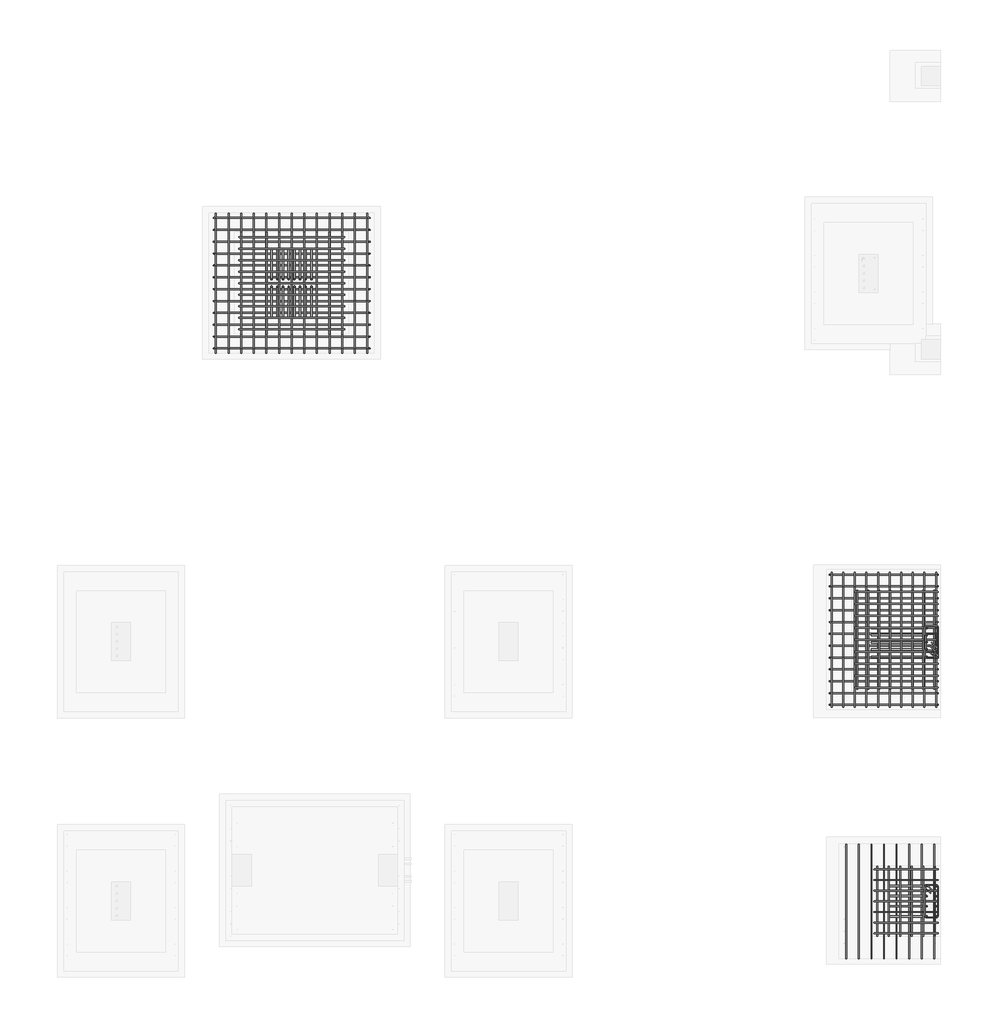
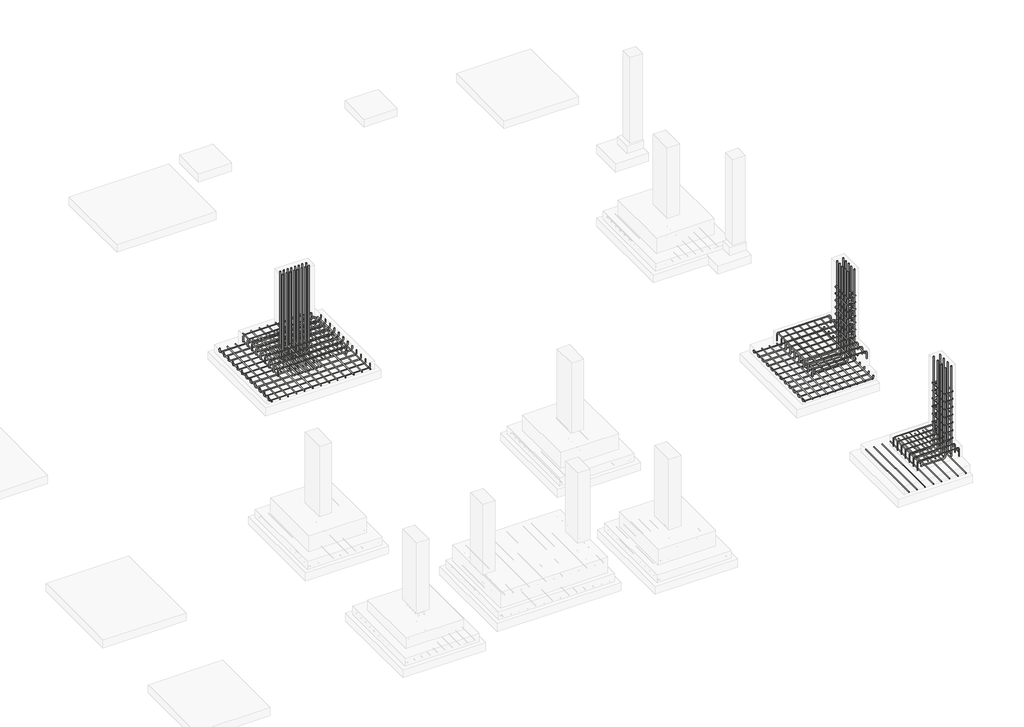
# One storey, part 5 of 6: 20 reinforcing bars.
"""IFC4 building model written with IfcOpenShell, lengths in millimetres."""

from ifc_helpers import new_model, si_unit, point, frame, origin, place, context, project, spatial, polyline, circle_curve, trimmed, segment, composite_curve, source, transform, mapped, element, save
from ifc_brep_helpers import swept_disk

model = new_model("IFC4")

# Units and contexts
model_context = context("Model", 3, world=origin())
ifc_project = project(units=[si_unit("LENGTHUNIT", "METRE", prefix="MILLI")], contexts=[model_context])

# Site, building, storey
site = spatial("IfcSite", under=ifc_project)
building = spatial("IfcBuilding", under=site)
storey = spatial("IfcBuildingStorey", under=building, Elevation=-1828.8)

# Reinforcing bars
placement = place(None, origin())
reinforcing_bar_shape = source(origin(), model_context, "Body", "SolidModel", [
    swept_disk(composite_curve([segment(polyline([(5676850.791013, -3593831.6523052, -1801.3373708), (5676850.791013, -3595448.0523052, -1801.3373708)]), True, "CONTINUOUS")], self_intersect=False), 6.0),
])
element("IfcReinforcingBar", 1, at=placement, inside=storey, context=model_context, shape_type="MappedRepresentation", body=[
    mapped(reinforcing_bar_shape, transform((0.0, 0.0, 0.0), x_axis=(1.0, 0.0, 0.0), y_axis=(0.0, 1.0, 0.0), z_axis=(0.0, 0.0, 1.0))),
    mapped(reinforcing_bar_shape, transform((-139.1053792, 0.0, 0.0), x_axis=(1.0, 0.0, 0.0), y_axis=(0.0, 1.0, 0.0), z_axis=(0.0, 0.0, 1.0))),
    mapped(reinforcing_bar_shape, transform((-278.2107585, 0.0, 0.0), x_axis=(1.0, 0.0, 0.0), y_axis=(0.0, 1.0, 0.0), z_axis=(0.0, 0.0, 1.0))),
    mapped(reinforcing_bar_shape, transform((-417.3161377, 0.0, 0.0), x_axis=(1.0, 0.0, 0.0), y_axis=(0.0, 1.0, 0.0), z_axis=(0.0, 0.0, 1.0))),
    mapped(reinforcing_bar_shape, transform((-556.4215169, 0.0, 0.0), x_axis=(1.0, 0.0, 0.0), y_axis=(0.0, 1.0, 0.0), z_axis=(0.0, 0.0, 1.0))),
    mapped(reinforcing_bar_shape, transform((-695.5268961, 0.0, 0.0), x_axis=(1.0, 0.0, 0.0), y_axis=(0.0, 1.0, 0.0), z_axis=(0.0, 0.0, 1.0))),
    mapped(reinforcing_bar_shape, transform((-834.6322754, 0.0, 0.0), x_axis=(1.0, 0.0, 0.0), y_axis=(0.0, 1.0, 0.0), z_axis=(0.0, 0.0, 1.0))),
    mapped(reinforcing_bar_shape, transform((-973.7376546, 0.0, 0.0), x_axis=(1.0, 0.0, 0.0), y_axis=(0.0, 1.0, 0.0), z_axis=(0.0, 0.0, 1.0))),
    mapped(reinforcing_bar_shape, transform((-1112.8430338, 0.0, 0.0), x_axis=(1.0, 0.0, 0.0), y_axis=(0.0, 1.0, 0.0), z_axis=(0.0, 0.0, 1.0))),
    mapped(reinforcing_bar_shape, transform((-1251.9484131, 0.0, 0.0), x_axis=(1.0, 0.0, 0.0), y_axis=(0.0, 1.0, 0.0), z_axis=(0.0, 0.0, 1.0))),
])
reinforcing_bar_2_shape = source(origin(), model_context, "Body", "SolidModel", [
    swept_disk(composite_curve([segment(polyline([(5675879.3650571, -3595213.4523052, -1551.6), (5675879.3650571, -3595213.4523052, -1437.6)]), True, "CONTINUOUS"), segment(trimmed(circle_curve(frame((5675909.3650571, -3595213.4523052, -1437.6), z_axis=(0.0, 1.0, 0.0), x_axis=(-30.0, 0.0, 0.0)), 30.0), [point((5675879.3650571, -3595213.4523052, -1437.6))], [point((5675909.3650571, -3595213.4523052, -1407.6))], True, "CARTESIAN"), True, "CONTINUOUS"), segment(polyline([(5675909.3650571, -3595213.4523052, -1407.6), (5676844.1650571, -3595213.4523052, -1407.6)]), True, "CONTINUOUS"), segment(trimmed(circle_curve(frame((5676844.1650571, -3595213.4523052, -1437.6), z_axis=(0.0, 1.0, 0.0), x_axis=(0.0, 0.0, 30.0)), 30.0), [point((5676844.1650571, -3595213.4523052, -1407.6))], [point((5676874.1650571, -3595213.4523052, -1437.6))], True, "CARTESIAN"), True, "CONTINUOUS"), segment(polyline([(5676874.1650571, -3595213.4523052, -1437.6), (5676874.1650571, -3595213.4523052, -1551.6)]), True, "CONTINUOUS")], self_intersect=False), 6.0),
])
element("IfcReinforcingBar", 2, at=placement, inside=storey, context=model_context, shape_type="MappedRepresentation", body=[
    mapped(reinforcing_bar_2_shape, transform((0.0, 0.0, 0.0), x_axis=(1.0, 0.0, 0.0), y_axis=(0.0, 1.0, 0.0), z_axis=(0.0, 0.0, 1.0))),
    mapped(reinforcing_bar_2_shape, transform((0.0, 143.4, 0.0), x_axis=(1.0, 0.0, 0.0), y_axis=(0.0, 1.0, 0.0), z_axis=(0.0, 0.0, 1.0))),
    mapped(reinforcing_bar_2_shape, transform((0.0, 286.8, 0.0), x_axis=(1.0, 0.0, 0.0), y_axis=(0.0, 1.0, 0.0), z_axis=(0.0, 0.0, 1.0))),
    mapped(reinforcing_bar_2_shape, transform((0.0, 430.2, 0.0), x_axis=(1.0, 0.0, 0.0), y_axis=(0.0, 1.0, 0.0), z_axis=(0.0, 0.0, 1.0))),
    mapped(reinforcing_bar_2_shape, transform((0.0, 573.6, 0.0), x_axis=(1.0, 0.0, 0.0), y_axis=(0.0, 1.0, 0.0), z_axis=(0.0, 0.0, 1.0))),
    mapped(reinforcing_bar_2_shape, transform((0.0, 717.0, 0.0), x_axis=(1.0, 0.0, 0.0), y_axis=(0.0, 1.0, 0.0), z_axis=(0.0, 0.0, 1.0))),
    mapped(reinforcing_bar_2_shape, transform((0.0, 860.4, 0.0), x_axis=(1.0, 0.0, 0.0), y_axis=(0.0, 1.0, 0.0), z_axis=(0.0, 0.0, 1.0))),
    mapped(reinforcing_bar_2_shape, transform((0.0, 1003.8, 0.0), x_axis=(1.0, 0.0, 0.0), y_axis=(0.0, 1.0, 0.0), z_axis=(0.0, 0.0, 1.0))),
    mapped(reinforcing_bar_2_shape, transform((0.0, 1147.2, 0.0), x_axis=(1.0, 0.0, 0.0), y_axis=(0.0, 1.0, 0.0), z_axis=(0.0, 0.0, 1.0))),
])
reinforcing_bar_3_shape = source(origin(), model_context, "Body", "SolidModel", [
    swept_disk(composite_curve([segment(polyline([(5675905.090534, -3595232.9223129, -1420.5088801), (5675905.090534, -3594045.3578875, -1420.5088801)]), True, "CONTINUOUS")], self_intersect=False), 6.0),
])
element("IfcReinforcingBar", 3, at=placement, inside=storey, context=model_context, shape_type="MappedRepresentation", body=[
    mapped(reinforcing_bar_3_shape, transform((0.0, 0.0, 0.0), x_axis=(1.0, 0.0, 0.0), y_axis=(0.0, 1.0, 0.0), z_axis=(0.0, 0.0, 1.0))),
    mapped(reinforcing_bar_3_shape, transform((131.8407277, 0.0, 0.0), x_axis=(1.0, 0.0, 0.0), y_axis=(0.0, 1.0, 0.0), z_axis=(0.0, 0.0, 1.0))),
    mapped(reinforcing_bar_3_shape, transform((263.6814554, 0.0, 0.0), x_axis=(1.0, 0.0, 0.0), y_axis=(0.0, 1.0, 0.0), z_axis=(0.0, 0.0, 1.0))),
    mapped(reinforcing_bar_3_shape, transform((395.5221831, 0.0, 0.0), x_axis=(1.0, 0.0, 0.0), y_axis=(0.0, 1.0, 0.0), z_axis=(0.0, 0.0, 1.0))),
    mapped(reinforcing_bar_3_shape, transform((527.3629109, 0.0, 0.0), x_axis=(1.0, 0.0, 0.0), y_axis=(0.0, 1.0, 0.0), z_axis=(0.0, 0.0, 1.0))),
    mapped(reinforcing_bar_3_shape, transform((659.2036386, 0.0, 0.0), x_axis=(1.0, 0.0, 0.0), y_axis=(0.0, 1.0, 0.0), z_axis=(0.0, 0.0, 1.0))),
    mapped(reinforcing_bar_3_shape, transform((791.0443663, 0.0, 0.0), x_axis=(1.0, 0.0, 0.0), y_axis=(0.0, 1.0, 0.0), z_axis=(0.0, 0.0, 1.0))),
    mapped(reinforcing_bar_3_shape, transform((922.885094, 0.0, 0.0), x_axis=(1.0, 0.0, 0.0), y_axis=(0.0, 1.0, 0.0), z_axis=(0.0, 0.0, 1.0))),
])
reinforcing_bar_4_shape = source(origin(), model_context, "Body", "SolidModel", [
    swept_disk(composite_curve([segment(polyline([(5675574.5650571, -3593858.3316435, -1763.0663631), (5675574.5650571, -3593858.3316435, -1784.4413329)]), True, "CONTINUOUS"), segment(trimmed(circle_curve(frame((5675604.5650571, -3593858.3316435, -1784.4413329), z_axis=(0.0, -1.0, 0.0), x_axis=(-30.0, 0.0, 0.0)), 30.0), [point((5675574.5650571, -3593858.3316435, -1784.4413329))], [point((5675604.5650571, -3593858.3316435, -1814.4413329))], True, "CARTESIAN"), True, "CONTINUOUS"), segment(polyline([(5675604.5650571, -3593858.3316435, -1814.4413329), (5676844.1650571, -3593858.3316435, -1814.4413329)]), True, "CONTINUOUS"), segment(trimmed(circle_curve(frame((5676844.1650571, -3593858.3316435, -1784.4413329), z_axis=(0.0, -1.0, 0.0), x_axis=(0.0, 0.0, -30.0)), 30.0), [point((5676844.1650571, -3593858.3316435, -1814.4413329))], [point((5676874.1650571, -3593858.3316435, -1784.4413329))], True, "CARTESIAN"), True, "CONTINUOUS"), segment(polyline([(5676874.1650571, -3593858.3316435, -1784.4413329), (5676874.1650571, -3593858.3316435, -1763.0663631)]), True, "CONTINUOUS")], self_intersect=False), 6.0),
])
element("IfcReinforcingBar", 4, at=placement, inside=storey, context=model_context, shape_type="MappedRepresentation", body=[
    mapped(reinforcing_bar_4_shape, transform((0.0, 0.0, 0.0), x_axis=(1.0, 0.0, 0.0), y_axis=(0.0, 1.0, 0.0), z_axis=(0.0, 0.0, 1.0))),
    mapped(reinforcing_bar_4_shape, transform((0.0, -142.0493969, 0.0), x_axis=(1.0, 0.0, 0.0), y_axis=(0.0, 1.0, 0.0), z_axis=(0.0, 0.0, 1.0))),
    mapped(reinforcing_bar_4_shape, transform((0.0, -284.0987939, 0.0), x_axis=(1.0, 0.0, 0.0), y_axis=(0.0, 1.0, 0.0), z_axis=(0.0, 0.0, 1.0))),
    mapped(reinforcing_bar_4_shape, transform((0.0, -426.1481908, 0.0), x_axis=(1.0, 0.0, 0.0), y_axis=(0.0, 1.0, 0.0), z_axis=(0.0, 0.0, 1.0))),
    mapped(reinforcing_bar_4_shape, transform((0.0, -568.1975878, 0.0), x_axis=(1.0, 0.0, 0.0), y_axis=(0.0, 1.0, 0.0), z_axis=(0.0, 0.0, 1.0))),
    mapped(reinforcing_bar_4_shape, transform((0.0, -710.2469847, 0.0), x_axis=(1.0, 0.0, 0.0), y_axis=(0.0, 1.0, 0.0), z_axis=(0.0, 0.0, 1.0))),
    mapped(reinforcing_bar_4_shape, transform((0.0, -852.2963817, 0.0), x_axis=(1.0, 0.0, 0.0), y_axis=(0.0, 1.0, 0.0), z_axis=(0.0, 0.0, 1.0))),
    mapped(reinforcing_bar_4_shape, transform((0.0, -994.3457786, 0.0), x_axis=(1.0, 0.0, 0.0), y_axis=(0.0, 1.0, 0.0), z_axis=(0.0, 0.0, 1.0))),
    mapped(reinforcing_bar_4_shape, transform((0.0, -1136.3951756, 0.0), x_axis=(1.0, 0.0, 0.0), y_axis=(0.0, 1.0, 0.0), z_axis=(0.0, 0.0, 1.0))),
    mapped(reinforcing_bar_4_shape, transform((0.0, -1278.4445725, 0.0), x_axis=(1.0, 0.0, 0.0), y_axis=(0.0, 1.0, 0.0), z_axis=(0.0, 0.0, 1.0))),
    mapped(reinforcing_bar_4_shape, transform((0.0, -1420.4939694, 0.0), x_axis=(1.0, 0.0, 0.0), y_axis=(0.0, 1.0, 0.0), z_axis=(0.0, 0.0, 1.0))),
    mapped(reinforcing_bar_4_shape, transform((0.0, -1562.5433664, 0.0), x_axis=(1.0, 0.0, 0.0), y_axis=(0.0, 1.0, 0.0), z_axis=(0.0, 0.0, 1.0))),
])
reinforcing_bar_5_shape = source(origin(), model_context, "Body", "SolidModel", [
    swept_disk(composite_curve([segment(polyline([(5675774.6470228, -3597090.2875145, -1807.7638193), (5675774.6470228, -3598461.8875145, -1807.7638193)]), True, "CONTINUOUS")], self_intersect=False), 5.0),
])
element("IfcReinforcingBar", 5, at=placement, inside=storey, context=model_context, shape_type="MappedRepresentation", body=[
    mapped(reinforcing_bar_5_shape, transform((0.0, 0.0, 0.0), x_axis=(1.0, 0.0, 0.0), y_axis=(0.0, 1.0, 0.0), z_axis=(0.0, 0.0, 1.0))),
    mapped(reinforcing_bar_5_shape, transform((150.6667583, 0.0, 0.0), x_axis=(1.0, 0.0, 0.0), y_axis=(0.0, 1.0, 0.0), z_axis=(0.0, 0.0, 1.0))),
    mapped(reinforcing_bar_5_shape, transform((301.3335165, 0.0, 0.0), x_axis=(1.0, 0.0, 0.0), y_axis=(0.0, 1.0, 0.0), z_axis=(0.0, 0.0, 1.0))),
    mapped(reinforcing_bar_5_shape, transform((452.0002748, 0.0, 0.0), x_axis=(1.0, 0.0, 0.0), y_axis=(0.0, 1.0, 0.0), z_axis=(0.0, 0.0, 1.0))),
    mapped(reinforcing_bar_5_shape, transform((602.6670331, 0.0, 0.0), x_axis=(1.0, 0.0, 0.0), y_axis=(0.0, 1.0, 0.0), z_axis=(0.0, 0.0, 1.0))),
    mapped(reinforcing_bar_5_shape, transform((753.3337913, 0.0, 0.0), x_axis=(1.0, 0.0, 0.0), y_axis=(0.0, 1.0, 0.0), z_axis=(0.0, 0.0, 1.0))),
    mapped(reinforcing_bar_5_shape, transform((904.0005496, 0.0, 0.0), x_axis=(1.0, 0.0, 0.0), y_axis=(0.0, 1.0, 0.0), z_axis=(0.0, 0.0, 1.0))),
    mapped(reinforcing_bar_5_shape, transform((1054.6673079, 0.0, 0.0), x_axis=(1.0, 0.0, 0.0), y_axis=(0.0, 1.0, 0.0), z_axis=(0.0, 0.0, 1.0))),
])
reinforcing_bar_6_shape = source(origin(), model_context, "Body", "SolidModel", [
    swept_disk(composite_curve([segment(polyline([(5676875.1650571, -3597391.9875145, -1673.2), (5676875.1650571, -3597391.9875145, -1533.2)]), True, "CONTINUOUS"), segment(trimmed(circle_curve(frame((5676850.1650571, -3597391.9875145, -1533.2), z_axis=(0.0, -1.0, 0.0), x_axis=(25.0, 0.0, 0.0)), 25.0), [point((5676875.1650571, -3597391.9875145, -1533.2))], [point((5676850.1650571, -3597391.9875145, -1508.2))], True, "CARTESIAN"), True, "CONTINUOUS"), segment(polyline([(5676850.1650571, -3597391.9875145, -1508.2), (5676131.9650571, -3597391.9875145, -1508.2)]), True, "CONTINUOUS"), segment(trimmed(circle_curve(frame((5676131.9650571, -3597391.9875145, -1533.2), z_axis=(0.0, -1.0, 0.0), x_axis=(0.0, 0.0, 25.0)), 25.0), [point((5676131.9650571, -3597391.9875145, -1508.2))], [point((5676106.9650571, -3597391.9875145, -1533.2))], True, "CARTESIAN"), True, "CONTINUOUS"), segment(polyline([(5676106.9650571, -3597391.9875145, -1533.2), (5676106.9650571, -3597391.9875145, -1673.2)]), True, "CONTINUOUS")], self_intersect=False), 5.0),
])
element("IfcReinforcingBar", 6, at=placement, inside=storey, context=model_context, shape_type="MappedRepresentation", body=[
    mapped(reinforcing_bar_6_shape, transform((0.0, 0.0, 0.0), x_axis=(1.0, 0.0, 0.0), y_axis=(0.0, 1.0, 0.0), z_axis=(0.0, 0.0, 1.0))),
    mapped(reinforcing_bar_6_shape, transform((0.0, -128.0333333, 0.0), x_axis=(1.0, 0.0, 0.0), y_axis=(0.0, 1.0, 0.0), z_axis=(0.0, 0.0, 1.0))),
    mapped(reinforcing_bar_6_shape, transform((0.0, -256.0666667, 0.0), x_axis=(1.0, 0.0, 0.0), y_axis=(0.0, 1.0, 0.0), z_axis=(0.0, 0.0, 1.0))),
    mapped(reinforcing_bar_6_shape, transform((0.0, -384.1, 0.0), x_axis=(1.0, 0.0, 0.0), y_axis=(0.0, 1.0, 0.0), z_axis=(0.0, 0.0, 1.0))),
    mapped(reinforcing_bar_6_shape, transform((0.0, -512.1333333, 0.0), x_axis=(1.0, 0.0, 0.0), y_axis=(0.0, 1.0, 0.0), z_axis=(0.0, 0.0, 1.0))),
    mapped(reinforcing_bar_6_shape, transform((0.0, -640.1666667, 0.0), x_axis=(1.0, 0.0, 0.0), y_axis=(0.0, 1.0, 0.0), z_axis=(0.0, 0.0, 1.0))),
    mapped(reinforcing_bar_6_shape, transform((0.0, -768.2, 0.0), x_axis=(1.0, 0.0, 0.0), y_axis=(0.0, 1.0, 0.0), z_axis=(0.0, 0.0, 1.0))),
])
reinforcing_bar_7_shape = source(origin(), model_context, "Body", "SolidModel", [
    swept_disk(composite_curve([segment(polyline([(5676837.7552182, -3597356.9875145, -1540.036299), (5676837.7552182, -3598195.1875145, -1540.036299)]), True, "CONTINUOUS")], self_intersect=False), 5.0),
])
element("IfcReinforcingBar", 7, at=placement, inside=storey, context=model_context, shape_type="MappedRepresentation", body=[
    mapped(reinforcing_bar_7_shape, transform((0.0, 0.0, 0.0), x_axis=(1.0, 0.0, 0.0), y_axis=(0.0, 1.0, 0.0), z_axis=(0.0, 0.0, 1.0))),
    mapped(reinforcing_bar_7_shape, transform((-138.6844386, 0.0, 0.0), x_axis=(1.0, 0.0, 0.0), y_axis=(0.0, 1.0, 0.0), z_axis=(0.0, 0.0, 1.0))),
    mapped(reinforcing_bar_7_shape, transform((-277.3688772, 0.0, 0.0), x_axis=(1.0, 0.0, 0.0), y_axis=(0.0, 1.0, 0.0), z_axis=(0.0, 0.0, 1.0))),
    mapped(reinforcing_bar_7_shape, transform((-416.0533158, 0.0, 0.0), x_axis=(1.0, 0.0, 0.0), y_axis=(0.0, 1.0, 0.0), z_axis=(0.0, 0.0, 1.0))),
    mapped(reinforcing_bar_7_shape, transform((-554.7377544, 0.0, 0.0), x_axis=(1.0, 0.0, 0.0), y_axis=(0.0, 1.0, 0.0), z_axis=(0.0, 0.0, 1.0))),
    mapped(reinforcing_bar_7_shape, transform((-693.422193, 0.0, 0.0), x_axis=(1.0, 0.0, 0.0), y_axis=(0.0, 1.0, 0.0), z_axis=(0.0, 0.0, 1.0))),
])
reinforcing_bar_8_shape = source(origin(), model_context, "Body", "SolidModel", [
    swept_disk(composite_curve([segment(polyline([(5668190.4297535, -3589581.8284482, -1732.3211603), (5668190.4297535, -3589581.8284482, -1781.3211603)]), True, "CONTINUOUS"), segment(trimmed(circle_curve(frame((5668220.4297535, -3589581.8284482, -1781.3211603), z_axis=(0.0, -1.0, 0.0), x_axis=(-30.0, 0.0, 0.0)), 30.0), [point((5668190.4297535, -3589581.8284482, -1781.3211603))], [point((5668220.4297535, -3589581.8284482, -1811.3211603))], True, "CARTESIAN"), True, "CONTINUOUS"), segment(polyline([(5668220.4297535, -3589581.8284482, -1811.3211603), (5670029.6297535, -3589581.8284482, -1811.3211603)]), True, "CONTINUOUS"), segment(trimmed(circle_curve(frame((5670029.6297535, -3589581.8284482, -1781.3211603), z_axis=(0.0, -1.0, 0.0), x_axis=(0.0, 0.0, -30.0)), 30.0), [point((5670029.6297535, -3589581.8284482, -1811.3211603))], [point((5670059.6297535, -3589581.8284482, -1781.3211603))], True, "CARTESIAN"), True, "CONTINUOUS"), segment(polyline([(5670059.6297535, -3589581.8284482, -1781.3211603), (5670059.6297535, -3589581.8284482, -1732.3211603)]), True, "CONTINUOUS")], self_intersect=False), 6.0),
])
element("IfcReinforcingBar", 8, at=placement, inside=storey, context=model_context, shape_type="MappedRepresentation", body=[
    mapped(reinforcing_bar_8_shape, transform((0.0, 0.0, 0.0), x_axis=(1.0, 0.0, 0.0), y_axis=(0.0, 1.0, 0.0), z_axis=(0.0, 0.0, 1.0))),
    mapped(reinforcing_bar_8_shape, transform((0.0, -142.2181818, 0.0), x_axis=(1.0, 0.0, 0.0), y_axis=(0.0, 1.0, 0.0), z_axis=(0.0, 0.0, 1.0))),
    mapped(reinforcing_bar_8_shape, transform((0.0, -284.4363636, 0.0), x_axis=(1.0, 0.0, 0.0), y_axis=(0.0, 1.0, 0.0), z_axis=(0.0, 0.0, 1.0))),
    mapped(reinforcing_bar_8_shape, transform((0.0, -426.6545455, 0.0), x_axis=(1.0, 0.0, 0.0), y_axis=(0.0, 1.0, 0.0), z_axis=(0.0, 0.0, 1.0))),
    mapped(reinforcing_bar_8_shape, transform((0.0, -568.8727273, 0.0), x_axis=(1.0, 0.0, 0.0), y_axis=(0.0, 1.0, 0.0), z_axis=(0.0, 0.0, 1.0))),
    mapped(reinforcing_bar_8_shape, transform((0.0, -711.0909091, 0.0), x_axis=(1.0, 0.0, 0.0), y_axis=(0.0, 1.0, 0.0), z_axis=(0.0, 0.0, 1.0))),
    mapped(reinforcing_bar_8_shape, transform((0.0, -853.3090909, 0.0), x_axis=(1.0, 0.0, 0.0), y_axis=(0.0, 1.0, 0.0), z_axis=(0.0, 0.0, 1.0))),
    mapped(reinforcing_bar_8_shape, transform((0.0, -995.5272727, 0.0), x_axis=(1.0, 0.0, 0.0), y_axis=(0.0, 1.0, 0.0), z_axis=(0.0, 0.0, 1.0))),
    mapped(reinforcing_bar_8_shape, transform((0.0, -1137.7454545, 0.0), x_axis=(1.0, 0.0, 0.0), y_axis=(0.0, 1.0, 0.0), z_axis=(0.0, 0.0, 1.0))),
    mapped(reinforcing_bar_8_shape, transform((0.0, -1279.9636364, 0.0), x_axis=(1.0, 0.0, 0.0), y_axis=(0.0, 1.0, 0.0), z_axis=(0.0, 0.0, 1.0))),
    mapped(reinforcing_bar_8_shape, transform((0.0, -1422.1818182, 0.0), x_axis=(1.0, 0.0, 0.0), y_axis=(0.0, 1.0, 0.0), z_axis=(0.0, 0.0, 1.0))),
    mapped(reinforcing_bar_8_shape, transform((0.0, -1564.4, 0.0), x_axis=(1.0, 0.0, 0.0), y_axis=(0.0, 1.0, 0.0), z_axis=(0.0, 0.0, 1.0))),
])
reinforcing_bar_9_shape = source(origin(), model_context, "Body", "SolidModel", [
    swept_disk(composite_curve([segment(polyline([(5669754.8297535, -3589810.4284482, -1571.6), (5669754.8297535, -3589810.4284482, -1472.0496054)]), True, "CONTINUOUS"), segment(trimmed(circle_curve(frame((5669724.8297535, -3589810.4284482, -1472.0496054), z_axis=(0.0, -1.0, 0.0), x_axis=(30.0, 0.0, 0.0)), 30.0), [point((5669754.8297535, -3589810.4284482, -1472.0496054))], [point((5669724.8297535, -3589810.4284482, -1442.0496054))], True, "CARTESIAN"), True, "CONTINUOUS"), segment(polyline([(5669724.8297535, -3589810.4284482, -1442.0496054), (5668525.2297535, -3589810.4284482, -1442.0496054)]), True, "CONTINUOUS"), segment(trimmed(circle_curve(frame((5668525.2297535, -3589810.4284482, -1472.0496054), z_axis=(0.0, -1.0, 0.0), x_axis=(0.0, 0.0, 30.0)), 30.0), [point((5668525.2297535, -3589810.4284482, -1442.0496054))], [point((5668495.2297535, -3589810.4284482, -1472.0496054))], True, "CARTESIAN"), True, "CONTINUOUS"), segment(polyline([(5668495.2297535, -3589810.4284482, -1472.0496054), (5668495.2297535, -3589810.4284482, -1571.6)]), True, "CONTINUOUS")], self_intersect=False), 6.0),
])
element("IfcReinforcingBar", 9, at=placement, inside=storey, context=model_context, shape_type="MappedRepresentation", body=[
    mapped(reinforcing_bar_9_shape, transform((0.0, 0.0, 0.0), x_axis=(1.0, 0.0, 0.0), y_axis=(0.0, 1.0, 0.0), z_axis=(0.0, 0.0, 1.0))),
    mapped(reinforcing_bar_9_shape, transform((0.0, -138.4, 0.0), x_axis=(1.0, 0.0, 0.0), y_axis=(0.0, 1.0, 0.0), z_axis=(0.0, 0.0, 1.0))),
    mapped(reinforcing_bar_9_shape, transform((0.0, -276.8, 0.0), x_axis=(1.0, 0.0, 0.0), y_axis=(0.0, 1.0, 0.0), z_axis=(0.0, 0.0, 1.0))),
    mapped(reinforcing_bar_9_shape, transform((0.0, -415.2, 0.0), x_axis=(1.0, 0.0, 0.0), y_axis=(0.0, 1.0, 0.0), z_axis=(0.0, 0.0, 1.0))),
    mapped(reinforcing_bar_9_shape, transform((0.0, -553.6, 0.0), x_axis=(1.0, 0.0, 0.0), y_axis=(0.0, 1.0, 0.0), z_axis=(0.0, 0.0, 1.0))),
    mapped(reinforcing_bar_9_shape, transform((0.0, -692.0, 0.0), x_axis=(1.0, 0.0, 0.0), y_axis=(0.0, 1.0, 0.0), z_axis=(0.0, 0.0, 1.0))),
    mapped(reinforcing_bar_9_shape, transform((0.0, -830.4, 0.0), x_axis=(1.0, 0.0, 0.0), y_axis=(0.0, 1.0, 0.0), z_axis=(0.0, 0.0, 1.0))),
    mapped(reinforcing_bar_9_shape, transform((0.0, -968.8, 0.0), x_axis=(1.0, 0.0, 0.0), y_axis=(0.0, 1.0, 0.0), z_axis=(0.0, 0.0, 1.0))),
    mapped(reinforcing_bar_9_shape, transform((0.0, -1107.2, 0.0), x_axis=(1.0, 0.0, 0.0), y_axis=(0.0, 1.0, 0.0), z_axis=(0.0, 0.0, 1.0))),
])
reinforcing_bar_10_shape = source(origin(), model_context, "Body", "SolidModel", [
    swept_disk(composite_curve([segment(polyline([(5668215.5822153, -3589525.8284482, -1797.8515506), (5668215.5822153, -3591202.2284482, -1797.8515506)]), True, "CONTINUOUS")], self_intersect=False), 6.0),
])
element("IfcReinforcingBar", 10, at=placement, inside=storey, context=model_context, shape_type="MappedRepresentation", body=[
    mapped(reinforcing_bar_10_shape, transform((0.0, 0.0, 0.0), x_axis=(1.0, 0.0, 0.0), y_axis=(0.0, 1.0, 0.0), z_axis=(0.0, 0.0, 1.0))),
    mapped(reinforcing_bar_10_shape, transform((151.368303, 0.0, 0.0), x_axis=(1.0, 0.0, 0.0), y_axis=(0.0, 1.0, 0.0), z_axis=(0.0, 0.0, 1.0))),
    mapped(reinforcing_bar_10_shape, transform((302.736606, 0.0, 0.0), x_axis=(1.0, 0.0, 0.0), y_axis=(0.0, 1.0, 0.0), z_axis=(0.0, 0.0, 1.0))),
    mapped(reinforcing_bar_10_shape, transform((454.104909, 0.0, 0.0), x_axis=(1.0, 0.0, 0.0), y_axis=(0.0, 1.0, 0.0), z_axis=(0.0, 0.0, 1.0))),
    mapped(reinforcing_bar_10_shape, transform((605.473212, 0.0, 0.0), x_axis=(1.0, 0.0, 0.0), y_axis=(0.0, 1.0, 0.0), z_axis=(0.0, 0.0, 1.0))),
    mapped(reinforcing_bar_10_shape, transform((756.841515, 0.0, 0.0), x_axis=(1.0, 0.0, 0.0), y_axis=(0.0, 1.0, 0.0), z_axis=(0.0, 0.0, 1.0))),
    mapped(reinforcing_bar_10_shape, transform((908.209818, 0.0, 0.0), x_axis=(1.0, 0.0, 0.0), y_axis=(0.0, 1.0, 0.0), z_axis=(0.0, 0.0, 1.0))),
    mapped(reinforcing_bar_10_shape, transform((1059.578121, 0.0, 0.0), x_axis=(1.0, 0.0, 0.0), y_axis=(0.0, 1.0, 0.0), z_axis=(0.0, 0.0, 1.0))),
    mapped(reinforcing_bar_10_shape, transform((1210.946424, 0.0, 0.0), x_axis=(1.0, 0.0, 0.0), y_axis=(0.0, 1.0, 0.0), z_axis=(0.0, 0.0, 1.0))),
    mapped(reinforcing_bar_10_shape, transform((1362.314727, 0.0, 0.0), x_axis=(1.0, 0.0, 0.0), y_axis=(0.0, 1.0, 0.0), z_axis=(0.0, 0.0, 1.0))),
    mapped(reinforcing_bar_10_shape, transform((1513.6830301, 0.0, 0.0), x_axis=(1.0, 0.0, 0.0), y_axis=(0.0, 1.0, 0.0), z_axis=(0.0, 0.0, 1.0))),
    mapped(reinforcing_bar_10_shape, transform((1665.0513331, 0.0, 0.0), x_axis=(1.0, 0.0, 0.0), y_axis=(0.0, 1.0, 0.0), z_axis=(0.0, 0.0, 1.0))),
    mapped(reinforcing_bar_10_shape, transform((1816.4196361, 0.0, 0.0), x_axis=(1.0, 0.0, 0.0), y_axis=(0.0, 1.0, 0.0), z_axis=(0.0, 0.0, 1.0))),
])
reinforcing_bar_11_shape = source(origin(), model_context, "Body", "SolidModel", [
    swept_disk(composite_curve([segment(polyline([(5669728.1085568, -3589754.4284482, -1454.2512323), (5669728.1085568, -3590973.6284482, -1454.2512323)]), True, "CONTINUOUS")], self_intersect=False), 6.0),
])
element("IfcReinforcingBar", 11, at=placement, inside=storey, context=model_context, shape_type="MappedRepresentation", body=[
    mapped(reinforcing_bar_11_shape, transform((0.0, 0.0, 0.0), x_axis=(1.0, 0.0, 0.0), y_axis=(0.0, 1.0, 0.0), z_axis=(0.0, 0.0, 1.0))),
    mapped(reinforcing_bar_11_shape, transform((-150.8576206, 0.0, 0.0), x_axis=(1.0, 0.0, 0.0), y_axis=(0.0, 1.0, 0.0), z_axis=(0.0, 0.0, 1.0))),
    mapped(reinforcing_bar_11_shape, transform((-301.7152411, 0.0, 0.0), x_axis=(1.0, 0.0, 0.0), y_axis=(0.0, 1.0, 0.0), z_axis=(0.0, 0.0, 1.0))),
    mapped(reinforcing_bar_11_shape, transform((-452.5728617, 0.0, 0.0), x_axis=(1.0, 0.0, 0.0), y_axis=(0.0, 1.0, 0.0), z_axis=(0.0, 0.0, 1.0))),
    mapped(reinforcing_bar_11_shape, transform((-603.4304823, 0.0, 0.0), x_axis=(1.0, 0.0, 0.0), y_axis=(0.0, 1.0, 0.0), z_axis=(0.0, 0.0, 1.0))),
    mapped(reinforcing_bar_11_shape, transform((-754.2881028, 0.0, 0.0), x_axis=(1.0, 0.0, 0.0), y_axis=(0.0, 1.0, 0.0), z_axis=(0.0, 0.0, 1.0))),
    mapped(reinforcing_bar_11_shape, transform((-905.1457234, 0.0, 0.0), x_axis=(1.0, 0.0, 0.0), y_axis=(0.0, 1.0, 0.0), z_axis=(0.0, 0.0, 1.0))),
    mapped(reinforcing_bar_11_shape, transform((-1056.003344, 0.0, 0.0), x_axis=(1.0, 0.0, 0.0), y_axis=(0.0, 1.0, 0.0), z_axis=(0.0, 0.0, 1.0))),
    mapped(reinforcing_bar_11_shape, transform((-1206.8609645, 0.0, 0.0), x_axis=(1.0, 0.0, 0.0), y_axis=(0.0, 1.0, 0.0), z_axis=(0.0, 0.0, 1.0))),
])
reinforcing_bar_12_shape = source(origin(), model_context, "Body", "SolidModel", [
    swept_disk(composite_curve([segment(polyline([(5676777.6762044, -3594789.6477237, -1337.6), (5676842.0229215, -3594853.9944408, -1337.6)]), True, "CONTINUOUS"), segment(trimmed(circle_curve(frame((5676856.1650571, -3594839.8523052, -1337.6), z_axis=(0.0, 0.0, 1.0), x_axis=(-14.142135600559413, -14.142135600093752, 0.0)), 20.0), [point((5676842.0229215, -3594853.9944408, -1337.6))], [point((5676876.1650571, -3594839.8523052, -1337.6))], True, "CARTESIAN"), True, "CONTINUOUS"), segment(polyline([(5676876.1650571, -3594839.8523052, -1337.6), (5676876.1650571, -3594490.6523052, -1337.6)]), True, "CONTINUOUS"), segment(trimmed(circle_curve(frame((5676856.1650571, -3594490.6523052, -1337.6), z_axis=(0.0, 0.0, 1.0), x_axis=(20.0, 0.0, 0.0)), 20.0), [point((5676876.1650571, -3594490.6523052, -1337.6))], [point((5676856.1650571, -3594470.6523052, -1337.6))], True, "CARTESIAN"), True, "CONTINUOUS"), segment(polyline([(5676856.1650571, -3594470.6523052, -1337.6), (5676735.5650571, -3594470.6523052, -1337.6)]), True, "CONTINUOUS"), segment(trimmed(circle_curve(frame((5676735.5650571, -3594490.6480815, -1338.0110129), z_axis=(0.0, -0.020550643642738037, 0.9997888132230072), x_axis=(0.0, 19.995776299852878, 0.41101290000005974)), 20.0), [point((5676735.5650571, -3594470.6523052, -1337.6))], [point((5676715.5650571, -3594490.6480815, -1338.0110129))], True, "CARTESIAN"), True, "CONTINUOUS"), segment(polyline([(5676715.5650571, -3594490.6480815, -1338.0110129), (5676715.5650571, -3594839.8565289, -1345.1889871)]), True, "CONTINUOUS"), segment(trimmed(circle_curve(frame((5676735.5650571, -3594839.8565289, -1345.1889871), z_axis=(0.0, -0.020550643642738037, 0.9997888132230072), x_axis=(-20.0, 0.0, 0.0)), 20.0), [point((5676715.5650571, -3594839.8565289, -1345.1889871))], [point((5676735.5650571, -3594859.8523052, -1345.6))], True, "CARTESIAN"), True, "CONTINUOUS"), segment(polyline([(5676735.5650571, -3594859.8523052, -1345.6), (5676856.1650571, -3594859.8523052, -1345.6)]), True, "CONTINUOUS"), segment(trimmed(circle_curve(frame((5676856.1650571, -3594839.8523052, -1345.6), z_axis=(0.0, 0.0, 1.0), x_axis=(0.0, -20.0, 0.0)), 20.0), [point((5676856.1650571, -3594859.8523052, -1345.6))], [point((5676870.3071927, -3594825.7101696, -1345.6))], True, "CARTESIAN"), True, "CONTINUOUS"), segment(polyline([(5676870.3071927, -3594825.7101696, -1345.6), (5676805.9604756, -3594761.3634525, -1345.6)]), True, "CONTINUOUS")], self_intersect=False), 4.0),
])
element("IfcReinforcingBar", 12, at=placement, inside=storey, context=model_context, shape_type="MappedRepresentation", body=[
    mapped(reinforcing_bar_12_shape, transform((0.0, 0.0, 0.0), x_axis=(1.0, 0.0, 0.0), y_axis=(0.0, 1.0, 0.0), z_axis=(0.0, 0.0, 1.0))),
    mapped(reinforcing_bar_12_shape, transform((0.0, 0.0, 132.5005059), x_axis=(1.0, 0.0, 0.0), y_axis=(0.0, 1.0, 0.0), z_axis=(0.0, 0.0, 1.0))),
    mapped(reinforcing_bar_12_shape, transform((0.0, 0.0, 265.0010117), x_axis=(1.0, 0.0, 0.0), y_axis=(0.0, 1.0, 0.0), z_axis=(0.0, 0.0, 1.0))),
    mapped(reinforcing_bar_12_shape, transform((0.0, 0.0, 397.5015176), x_axis=(1.0, 0.0, 0.0), y_axis=(0.0, 1.0, 0.0), z_axis=(0.0, 0.0, 1.0))),
    mapped(reinforcing_bar_12_shape, transform((0.0, 0.0, 530.0020234), x_axis=(1.0, 0.0, 0.0), y_axis=(0.0, 1.0, 0.0), z_axis=(0.0, 0.0, 1.0))),
    mapped(reinforcing_bar_12_shape, transform((0.0, 0.0, 662.5025293), x_axis=(1.0, 0.0, 0.0), y_axis=(0.0, 1.0, 0.0), z_axis=(0.0, 0.0, 1.0))),
    mapped(reinforcing_bar_12_shape, transform((0.0, 0.0, 795.0030351), x_axis=(1.0, 0.0, 0.0), y_axis=(0.0, 1.0, 0.0), z_axis=(0.0, 0.0, 1.0))),
])
reinforcing_bar_13_shape = source(origin(), model_context, "Body", "SolidModel", [
    swept_disk(composite_curve([segment(polyline([(5676767.4306572, -3594701.6418417, -1337.6), (5676831.7773743, -3594765.9885587, -1337.6)]), True, "CONTINUOUS"), segment(trimmed(circle_curve(frame((5676845.9195099, -3594751.8464231, -1337.6), z_axis=(0.0, 0.0, 1.0), x_axis=(-14.14213559962809, -14.14213559962809, 0.0)), 20.0), [point((5676831.7773743, -3594765.9885587, -1337.6))], [point((5676865.9195099, -3594751.8464231, -1337.6))], True, "CARTESIAN"), True, "CONTINUOUS"), segment(polyline([(5676865.9195099, -3594751.8464231, -1337.6), (5676865.9195099, -3594584.8967698, -1337.6)]), True, "CONTINUOUS"), segment(trimmed(circle_curve(frame((5676845.9195099, -3594584.8967698, -1337.6), z_axis=(0.0, 0.0, 1.0), x_axis=(20.0, 0.0, 0.0)), 20.0), [point((5676865.9195099, -3594584.8967698, -1337.6))], [point((5676845.9195099, -3594564.8967698, -1337.6))], True, "CARTESIAN"), True, "CONTINUOUS"), segment(polyline([(5676845.9195099, -3594564.8967698, -1337.6), (5676747.2709985, -3594564.8967698, -1337.6)]), True, "CONTINUOUS"), segment(trimmed(circle_curve(frame((5676747.2709985, -3594584.881843, -1338.3725579), z_axis=(0.0, -0.038627894201681265, 0.9992536643863478), x_axis=(0.0, 19.985073199961334, 0.772557900000038)), 20.0), [point((5676747.2709985, -3594564.8967698, -1337.6))], [point((5676727.2709985, -3594584.881843, -1338.3725579))], True, "CARTESIAN"), True, "CONTINUOUS"), segment(polyline([(5676727.2709985, -3594584.881843, -1338.3725579), (5676727.2709985, -3594751.8613498, -1344.8274421)]), True, "CONTINUOUS"), segment(trimmed(circle_curve(frame((5676747.2709985, -3594751.8613498, -1344.8274421), z_axis=(0.0, -0.038627894201681265, 0.9992536643863478), x_axis=(-20.0, 0.0, 0.0)), 20.0), [point((5676727.2709985, -3594751.8613498, -1344.8274421))], [point((5676747.2709985, -3594771.8464231, -1345.6))], True, "CARTESIAN"), True, "CONTINUOUS"), segment(polyline([(5676747.2709985, -3594771.8464231, -1345.6), (5676845.9195099, -3594771.8464231, -1345.6)]), True, "CONTINUOUS"), segment(trimmed(circle_curve(frame((5676845.9195099, -3594751.8464231, -1345.6), z_axis=(0.0, 0.0, 1.0), x_axis=(0.0, -20.0, 0.0)), 20.0), [point((5676845.9195099, -3594771.8464231, -1345.6))], [point((5676860.0616455, -3594737.7042875, -1345.6))], True, "CARTESIAN"), True, "CONTINUOUS"), segment(polyline([(5676860.0616455, -3594737.7042875, -1345.6), (5676795.7149285, -3594673.3575704, -1345.6)]), True, "CONTINUOUS")], self_intersect=False), 4.0),
])
element("IfcReinforcingBar", 13, at=placement, inside=storey, context=model_context, shape_type="MappedRepresentation", body=[
    mapped(reinforcing_bar_13_shape, transform((0.0, 0.0, 0.0), x_axis=(1.0, 0.0, 0.0), y_axis=(0.0, 1.0, 0.0), z_axis=(0.0, 0.0, 1.0))),
    mapped(reinforcing_bar_13_shape, transform((0.0, 0.0, 132.5005059), x_axis=(1.0, 0.0, 0.0), y_axis=(0.0, 1.0, 0.0), z_axis=(0.0, 0.0, 1.0))),
    mapped(reinforcing_bar_13_shape, transform((0.0, 0.0, 265.0010117), x_axis=(1.0, 0.0, 0.0), y_axis=(0.0, 1.0, 0.0), z_axis=(0.0, 0.0, 1.0))),
    mapped(reinforcing_bar_13_shape, transform((0.0, 0.0, 397.5015176), x_axis=(1.0, 0.0, 0.0), y_axis=(0.0, 1.0, 0.0), z_axis=(0.0, 0.0, 1.0))),
    mapped(reinforcing_bar_13_shape, transform((0.0, 0.0, 530.0020234), x_axis=(1.0, 0.0, 0.0), y_axis=(0.0, 1.0, 0.0), z_axis=(0.0, 0.0, 1.0))),
    mapped(reinforcing_bar_13_shape, transform((0.0, 0.0, 662.5025293), x_axis=(1.0, 0.0, 0.0), y_axis=(0.0, 1.0, 0.0), z_axis=(0.0, 0.0, 1.0))),
    mapped(reinforcing_bar_13_shape, transform((0.0, 0.0, 795.0030351), x_axis=(1.0, 0.0, 0.0), y_axis=(0.0, 1.0, 0.0), z_axis=(0.0, 0.0, 1.0))),
])
reinforcing_bar_14_shape = source(origin(), model_context, "Body", "SolidModel", [
    swept_disk(composite_curve([segment(polyline([(5676739.2709985, -3594497.7254596, -40.0), (5676739.2709985, -3594497.7254596, -1746.25)]), True, "CONTINUOUS"), segment(trimmed(circle_curve(frame((5676699.2709985, -3594497.7254596, -1746.25), z_axis=(0.0, 1.0, 0.0), x_axis=(40.0, 0.0, 0.0)), 40.0), [point((5676739.2709985, -3594497.7254596, -1746.25))], [point((5676699.2709985, -3594497.7254596, -1786.25))], True, "CARTESIAN"), True, "CONTINUOUS"), segment(polyline([(5676699.2709985, -3594497.7254596, -1786.25), (5676071.8567351, -3594497.7254596, -1786.25)]), True, "CONTINUOUS")], self_intersect=False), 8.0),
])
element("IfcReinforcingBar", 14, at=placement, inside=storey, context=model_context, shape_type="MappedRepresentation", body=[
    mapped(reinforcing_bar_14_shape, transform((0.0, 0.0, 0.0), x_axis=(1.0, 0.0, 0.0), y_axis=(0.0, 1.0, 0.0), z_axis=(0.0, 0.0, 1.0))),
    mapped(reinforcing_bar_14_shape, transform((0.0, -86.3, 0.0), x_axis=(1.0, 0.0, 0.0), y_axis=(0.0, 1.0, 0.0), z_axis=(0.0, 0.0, 1.0))),
    mapped(reinforcing_bar_14_shape, transform((0.0, -172.6, 0.0), x_axis=(1.0, 0.0, 0.0), y_axis=(0.0, 1.0, 0.0), z_axis=(0.0, 0.0, 1.0))),
    mapped(reinforcing_bar_14_shape, transform((0.0, -258.9, 0.0), x_axis=(1.0, 0.0, 0.0), y_axis=(0.0, 1.0, 0.0), z_axis=(0.0, 0.0, 1.0))),
    mapped(reinforcing_bar_14_shape, transform((0.0, -345.2, 0.0), x_axis=(1.0, 0.0, 0.0), y_axis=(0.0, 1.0, 0.0), z_axis=(0.0, 0.0, 1.0))),
])
reinforcing_bar_15_shape = source(origin(), model_context, "Body", "SolidModel", [
    swept_disk(composite_curve([segment(polyline([(5676856.1650571, -3594489.3930996, -30.0), (5676856.1650571, -3594489.3930996, -1787.5415145)]), True, "CONTINUOUS")], self_intersect=False), 8.0),
])
element("IfcReinforcingBar", 15, at=placement, inside=storey, context=model_context, shape_type="MappedRepresentation", body=[
    mapped(reinforcing_bar_15_shape, transform((0.0, 0.0, 0.0), x_axis=(1.0, 0.0, 0.0), y_axis=(0.0, 1.0, 0.0), z_axis=(0.0, 0.0, 1.0))),
    mapped(reinforcing_bar_15_shape, transform((0.0, -89.6148014, 0.0), x_axis=(1.0, 0.0, 0.0), y_axis=(0.0, 1.0, 0.0), z_axis=(0.0, 0.0, 1.0))),
    mapped(reinforcing_bar_15_shape, transform((0.0, -179.2296028, 0.0), x_axis=(1.0, 0.0, 0.0), y_axis=(0.0, 1.0, 0.0), z_axis=(0.0, 0.0, 1.0))),
    mapped(reinforcing_bar_15_shape, transform((0.0, -268.8444042, 0.0), x_axis=(1.0, 0.0, 0.0), y_axis=(0.0, 1.0, 0.0), z_axis=(0.0, 0.0, 1.0))),
    mapped(reinforcing_bar_15_shape, transform((0.0, -358.4592056, 0.0), x_axis=(1.0, 0.0, 0.0), y_axis=(0.0, 1.0, 0.0), z_axis=(0.0, 0.0, 1.0))),
])
reinforcing_bar_16_shape = source(origin(), model_context, "Body", "SolidModel", [
    swept_disk(composite_curve([segment(polyline([(5676814.00016, -3597650.1021568, -1439.2), (5676749.6534429, -3597585.7554398, -1439.2)]), True, "CONTINUOUS"), segment(trimmed(circle_curve(frame((5676735.5113073, -3597599.8975754, -1439.2), z_axis=(0.0, 0.0, 1.0), x_axis=(14.14213559962809, 14.14213559962809, 0.0)), 20.0), [point((5676749.6534429, -3597585.7554398, -1439.2))], [point((5676715.5113073, -3597599.8975754, -1439.2))], True, "CARTESIAN"), True, "CONTINUOUS"), segment(polyline([(5676715.5113073, -3597599.8975754, -1439.2), (5676715.5113073, -3597949.0975754, -1439.2)]), True, "CONTINUOUS"), segment(trimmed(circle_curve(frame((5676735.5113073, -3597949.0975754, -1439.2), z_axis=(0.0, 0.0, 1.0), x_axis=(-20.0, 0.0, 0.0)), 20.0), [point((5676715.5113073, -3597949.0975754, -1439.2))], [point((5676735.5113073, -3597969.0975754, -1439.2))], True, "CARTESIAN"), True, "CONTINUOUS"), segment(polyline([(5676735.5113073, -3597969.0975754, -1439.2), (5676856.1113073, -3597969.0975754, -1439.2)]), True, "CONTINUOUS"), segment(trimmed(circle_curve(frame((5676856.1113073, -3597949.1017991, -1439.6110129), z_axis=(0.0, 0.020550643642841034, 0.9997888132230052), x_axis=(0.0, -19.995776299852878, 0.41101290000005974)), 20.0), [point((5676856.1113073, -3597969.0975754, -1439.2))], [point((5676876.1113073, -3597949.1017991, -1439.6110129))], True, "CARTESIAN"), True, "CONTINUOUS"), segment(polyline([(5676876.1113073, -3597949.1017991, -1439.6110129), (5676876.1113073, -3597599.8933516, -1446.7889871)]), True, "CONTINUOUS"), segment(trimmed(circle_curve(frame((5676856.1113073, -3597599.8933516, -1446.7889871), z_axis=(0.0, 0.020550643642841034, 0.9997888132230052), x_axis=(20.0, 0.0, 0.0)), 20.0), [point((5676876.1113073, -3597599.8933516, -1446.7889871))], [point((5676856.1113073, -3597579.8975754, -1447.2))], True, "CARTESIAN"), True, "CONTINUOUS"), segment(polyline([(5676856.1113073, -3597579.8975754, -1447.2), (5676735.5113073, -3597579.8975754, -1447.2)]), True, "CONTINUOUS"), segment(trimmed(circle_curve(frame((5676735.5113073, -3597599.8975754, -1447.2), z_axis=(0.0, 0.0, 1.0), x_axis=(0.0, 20.0, 0.0)), 20.0), [point((5676735.5113073, -3597579.8975754, -1447.2))], [point((5676721.3691717, -3597614.039711, -1447.2))], True, "CARTESIAN"), True, "CONTINUOUS"), segment(polyline([(5676721.3691717, -3597614.039711, -1447.2), (5676785.7158888, -3597678.3864281, -1447.2)]), True, "CONTINUOUS")], self_intersect=False), 4.0),
])
element("IfcReinforcingBar", 16, at=placement, inside=storey, context=model_context, shape_type="MappedRepresentation", body=[
    mapped(reinforcing_bar_16_shape, transform((0.0, 0.0, 0.0), x_axis=(1.0, 0.0, 0.0), y_axis=(0.0, 1.0, 0.0), z_axis=(0.0, 0.0, 1.0))),
    mapped(reinforcing_bar_16_shape, transform((0.0, 0.0, 151.8808383), x_axis=(1.0, 0.0, 0.0), y_axis=(0.0, 1.0, 0.0), z_axis=(0.0, 0.0, 1.0))),
    mapped(reinforcing_bar_16_shape, transform((0.0, 0.0, 303.7616766), x_axis=(1.0, 0.0, 0.0), y_axis=(0.0, 1.0, 0.0), z_axis=(0.0, 0.0, 1.0))),
    mapped(reinforcing_bar_16_shape, transform((0.0, 0.0, 455.642515), x_axis=(1.0, 0.0, 0.0), y_axis=(0.0, 1.0, 0.0), z_axis=(0.0, 0.0, 1.0))),
    mapped(reinforcing_bar_16_shape, transform((0.0, 0.0, 607.5233533), x_axis=(1.0, 0.0, 0.0), y_axis=(0.0, 1.0, 0.0), z_axis=(0.0, 0.0, 1.0))),
    mapped(reinforcing_bar_16_shape, transform((0.0, 0.0, 759.4041916), x_axis=(1.0, 0.0, 0.0), y_axis=(0.0, 1.0, 0.0), z_axis=(0.0, 0.0, 1.0))),
    mapped(reinforcing_bar_16_shape, transform((0.0, 0.0, 911.2850299), x_axis=(1.0, 0.0, 0.0), y_axis=(0.0, 1.0, 0.0), z_axis=(0.0, 0.0, 1.0))),
])
reinforcing_bar_17_shape = source(origin(), model_context, "Body", "SolidModel", [
    swept_disk(composite_curve([segment(polyline([(5676738.6613073, -3597591.8975754, -30.0), (5676738.6613073, -3597591.8975754, -1742.6)]), True, "CONTINUOUS"), segment(trimmed(circle_curve(frame((5676698.6613073, -3597591.8975754, -1742.6), z_axis=(0.0, 1.0, 0.0), x_axis=(40.0, 0.0, 0.0)), 40.0), [point((5676738.6613073, -3597591.8975754, -1742.6))], [point((5676698.6613073, -3597591.8975754, -1782.6))], True, "CARTESIAN"), True, "CONTINUOUS"), segment(polyline([(5676698.6613073, -3597591.8975754, -1782.6), (5676294.1613073, -3597591.8975754, -1782.6)]), True, "CONTINUOUS")], self_intersect=False), 8.0),
])
element("IfcReinforcingBar", 17, at=placement, inside=storey, context=model_context, shape_type="MappedRepresentation", body=[
    mapped(reinforcing_bar_17_shape, transform((0.0, 0.0, 0.0), x_axis=(1.0, 0.0, 0.0), y_axis=(0.0, 1.0, 0.0), z_axis=(0.0, 0.0, 1.0))),
    mapped(reinforcing_bar_17_shape, transform((0.0, -121.7333333, 0.0), x_axis=(1.0, 0.0, 0.0), y_axis=(0.0, 1.0, 0.0), z_axis=(0.0, 0.0, 1.0))),
    mapped(reinforcing_bar_17_shape, transform((0.0, -243.4666667, 0.0), x_axis=(1.0, 0.0, 0.0), y_axis=(0.0, 1.0, 0.0), z_axis=(0.0, 0.0, 1.0))),
    mapped(reinforcing_bar_17_shape, transform((0.0, -365.2, 0.0), x_axis=(1.0, 0.0, 0.0), y_axis=(0.0, 1.0, 0.0), z_axis=(0.0, 0.0, 1.0))),
])
reinforcing_bar_18_shape = source(origin(), model_context, "Body", "SolidModel", [
    swept_disk(composite_curve([segment(polyline([(5676852.9613073, -3597594.6836876, -30.0), (5676852.9613073, -3597594.6836876, -1788.95)]), True, "CONTINUOUS")], self_intersect=False), 8.0),
])
element("IfcReinforcingBar", 18, at=placement, inside=storey, context=model_context, shape_type="MappedRepresentation", body=[
    mapped(reinforcing_bar_18_shape, transform((0.0, 0.0, 0.0), x_axis=(1.0, 0.0, 0.0), y_axis=(0.0, 1.0, 0.0), z_axis=(0.0, 0.0, 1.0))),
    mapped(reinforcing_bar_18_shape, transform((0.0, -120.1712362, 0.0), x_axis=(1.0, 0.0, 0.0), y_axis=(0.0, 1.0, 0.0), z_axis=(0.0, 0.0, 1.0))),
    mapped(reinforcing_bar_18_shape, transform((0.0, -240.3424723, 0.0), x_axis=(1.0, 0.0, 0.0), y_axis=(0.0, 1.0, 0.0), z_axis=(0.0, 0.0, 1.0))),
    mapped(reinforcing_bar_18_shape, transform((0.0, -360.5137085, 0.0), x_axis=(1.0, 0.0, 0.0), y_axis=(0.0, 1.0, 0.0), z_axis=(0.0, 0.0, 1.0))),
])
reinforcing_bar_19_shape = source(origin(), model_context, "Body", "SolidModel", [
    swept_disk(composite_curve([segment(polyline([(5668882.1753663, -3590316.6993753, -30.0), (5668882.1753663, -3590316.6993753, -1741.5470698)]), True, "CONTINUOUS"), segment(trimmed(circle_curve(frame((5668882.1547311, -3590276.6993806, -1741.5470698), z_axis=(0.999999866933986, 0.0005158798409588551, 0.0), x_axis=(0.02063519973307848, -39.99999470030889, 0.0)), 40.0), [point((5668882.1753663, -3590316.6993753, -1741.5470698))], [point((5668882.1547311, -3590276.6993806, -1781.5470698))], True, "CARTESIAN"), True, "CONTINUOUS"), segment(polyline([(5668882.1547311, -3590276.6993806, -1781.5470698), (5668881.9853678, -3589948.3994243, -1781.5470698)]), True, "CONTINUOUS")], self_intersect=False), 8.0),
])
element("IfcReinforcingBar", 19, at=placement, inside=storey, context=model_context, shape_type="MappedRepresentation", body=[
    mapped(reinforcing_bar_19_shape, transform((0.0, 0.0, 0.0), x_axis=(1.0, 0.0, 0.0), y_axis=(0.0, 1.0, 0.0), z_axis=(0.0, 0.0, 1.0))),
    mapped(reinforcing_bar_19_shape, transform((68.4918907, 0.0353336, 0.0), x_axis=(1.0, 0.0, 0.0), y_axis=(0.0, 1.0, 0.0), z_axis=(0.0, 0.0, 1.0))),
    mapped(reinforcing_bar_19_shape, transform((136.9837814, 0.0706672, 0.0), x_axis=(1.0, 0.0, 0.0), y_axis=(0.0, 1.0, 0.0), z_axis=(0.0, 0.0, 1.0))),
    mapped(reinforcing_bar_19_shape, transform((205.4756721, 0.1060008, 0.0), x_axis=(1.0, 0.0, 0.0), y_axis=(0.0, 1.0, 0.0), z_axis=(0.0, 0.0, 1.0))),
    mapped(reinforcing_bar_19_shape, transform((273.9675627, 0.1413344, 0.0), x_axis=(1.0, 0.0, 0.0), y_axis=(0.0, 1.0, 0.0), z_axis=(0.0, 0.0, 1.0))),
    mapped(reinforcing_bar_19_shape, transform((342.4594534, 0.176668, 0.0), x_axis=(1.0, 0.0, 0.0), y_axis=(0.0, 1.0, 0.0), z_axis=(0.0, 0.0, 1.0))),
    mapped(reinforcing_bar_19_shape, transform((410.9513441, 0.2120015, 0.0), x_axis=(1.0, 0.0, 0.0), y_axis=(0.0, 1.0, 0.0), z_axis=(0.0, 0.0, 1.0))),
    mapped(reinforcing_bar_19_shape, transform((479.4432348, 0.2473351, 0.0), x_axis=(1.0, 0.0, 0.0), y_axis=(0.0, 1.0, 0.0), z_axis=(0.0, 0.0, 1.0))),
])
reinforcing_bar_20_shape = source(origin(), model_context, "Body", "SolidModel", [
    swept_disk(composite_curve([segment(polyline([(5668882.4321488, -3590404.887339, -30.0), (5668882.4321488, -3590404.887339, -1741.5470698)]), True, "CONTINUOUS"), segment(trimmed(circle_curve(frame((5668882.4115136, -3590444.8873337, -1741.5470698), z_axis=(-0.999999866933986, 0.0005158798409588551, 0.0), x_axis=(0.020635200664401054, 39.99999469984323, 0.0)), 40.0), [point((5668882.4321488, -3590404.887339, -1741.5470698))], [point((5668882.4115136, -3590444.8873337, -1781.5470698))], True, "CARTESIAN"), True, "CONTINUOUS"), segment(polyline([(5668882.4115136, -3590444.8873337, -1781.5470698), (5668882.2421502, -3590773.18729, -1781.5470698)]), True, "CONTINUOUS")], self_intersect=False), 8.0),
])
element("IfcReinforcingBar", 20, at=placement, inside=storey, context=model_context, shape_type="MappedRepresentation", body=[
    mapped(reinforcing_bar_20_shape, transform((0.0, 0.0, 0.0), x_axis=(1.0, 0.0, 0.0), y_axis=(0.0, 1.0, 0.0), z_axis=(0.0, 0.0, 1.0))),
    mapped(reinforcing_bar_20_shape, transform((68.4905243, -0.0353329, 0.0), x_axis=(1.0, 0.0, 0.0), y_axis=(0.0, 1.0, 0.0), z_axis=(0.0, 0.0, 1.0))),
    mapped(reinforcing_bar_20_shape, transform((136.9810486, -0.0706658, 0.0), x_axis=(1.0, 0.0, 0.0), y_axis=(0.0, 1.0, 0.0), z_axis=(0.0, 0.0, 1.0))),
    mapped(reinforcing_bar_20_shape, transform((205.4715729, -0.1059987, 0.0), x_axis=(1.0, 0.0, 0.0), y_axis=(0.0, 1.0, 0.0), z_axis=(0.0, 0.0, 1.0))),
    mapped(reinforcing_bar_20_shape, transform((273.9620972, -0.1413315, 0.0), x_axis=(1.0, 0.0, 0.0), y_axis=(0.0, 1.0, 0.0), z_axis=(0.0, 0.0, 1.0))),
    mapped(reinforcing_bar_20_shape, transform((342.4526215, -0.1766644, 0.0), x_axis=(1.0, 0.0, 0.0), y_axis=(0.0, 1.0, 0.0), z_axis=(0.0, 0.0, 1.0))),
    mapped(reinforcing_bar_20_shape, transform((410.9431458, -0.2119973, 0.0), x_axis=(1.0, 0.0, 0.0), y_axis=(0.0, 1.0, 0.0), z_axis=(0.0, 0.0, 1.0))),
    mapped(reinforcing_bar_20_shape, transform((479.4336701, -0.2473302, 0.0), x_axis=(1.0, 0.0, 0.0), y_axis=(0.0, 1.0, 0.0), z_axis=(0.0, 0.0, 1.0))),
])

save(model, "model.ifc")

# Revit data of these elements
# Elements 1, 2, 3, 4, 5, 6, 7, 8, 9, 10, 11, 12, 13, 14, 15, 16, 17, 18, 19, 20 (IfcReinforcingBar)
#   Phase Created = New Construction
